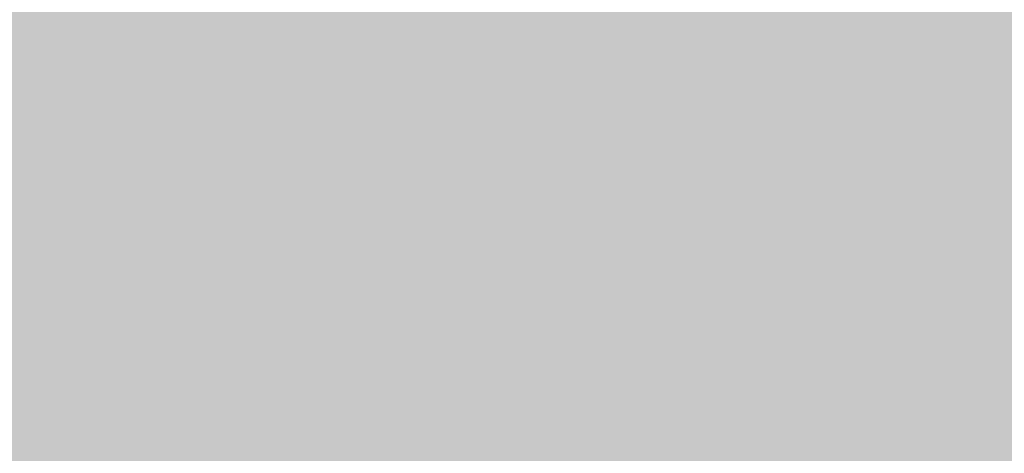
# Model space of a CAD drawing. Units: feet. Extents: x 3168 to 4724, y 827 to 1477.
# Tile 100 of 256: x 3277.376 to 3284.479, y 1093.654 to 1096.781. Entities that reach past the tile are written whole.
import ezdxf

# ---------------------------------------------------------------- set-up
doc = ezdxf.new("R2010")
doc.units = ezdxf.units.FT
doc.layers.add('A-ELEV-PATT', color=8, linetype='Continuous', lineweight=13)

msp = doc.modelspace()

# ---------------------------------------------------------------- hatches: boundary and pattern name
at = {"layer": 'A-ELEV-PATT'}
h = msp.add_hatch(color=256, dxfattribs=at)
h.dxf.hatch_style = 1
edge = h.paths.add_edge_path()
edge.add_ellipse((3552.9058, 979.2201), major_axis=(36.7449, 0), ratio=0.4848485, start_angle=0, end_angle=360)
edge = h.paths.add_edge_path()
edge.add_ellipse((3559.8916, 929.2523), major_axis=(36.7449, 0), ratio=0.4848485, start_angle=0, end_angle=360)
edge = h.paths.add_edge_path()
edge.add_line((3299.3168, 1198.6061), (3479.9167, 1198.6061))
edge.add_line((3479.9167, 1198.6061), (3479.9167, 1209.8686))
edge.add_spline(control_points=[(3479.9167, 1209.8686), (3464.3012, 1209.8686), (3448.6856, 1209.8686), (3410.9491, 1209.8686), (3388.8282, 1209.8686), (3355.6469, 1209.8686), (3344.5864, 1209.8686), (3327.9957, 1209.8686), (3322.4655, 1209.8686), (3314.1702, 1209.8686), (3311.4051, 1209.8686), (3307.2574, 1209.8686), (3305.8748, 1209.8686), (3303.801, 1209.8686), (3303.1097, 1209.8686), (3302.0728, 1209.8686), (3301.7272, 1209.8686), (3301.2087, 1209.8686), (3301.0359, 1209.8686), (3300.7767, 1209.8686), (3300.6903, 1209.8686), (3300.5606, 1209.8686), (3300.5174, 1209.8686), (3300.4526, 1209.8686), (3300.431, 1209.8686), (3300.3986, 1209.8686), (3300.3878, 1209.8686), (3300.3662, 1209.8686), (3300.3457, 1209.8686), (3300.3455, 1209.8686), (3300.3455, 1209.8686), (3300.3433, 1209.8686), (3300.3411, 1209.8686), (3300.3379, 1209.8686), (3300.3368, 1209.8686), (3300.3339, 1209.8686), (3300.3321, 1209.8686), (3300.3255, 1209.8686), (3300.3207, 1209.8686), (3300.3109, 1209.8686), (3300.306, 1209.8686), (3300.2905, 1209.8686), (3300.28, 1209.8686), (3300.2324, 1209.8688), (3300.1953, 1209.869), (3299.9511, 1209.8706), (3299.7448, 1209.8743), (3299.4368, 1209.8833), (3299.3344, 1209.8868), (3299.1811, 1209.8929), (3299.13, 1209.8951), (3298.6522, 1209.9168), (3298.2295, 1209.9457), (3297.6016, 1210.0024), (3297.3934, 1210.0235), (3297.0827, 1210.0583), (3296.9793, 1210.0705), (3296.293, 1210.1549), (3295.7181, 1210.2434), (3294.8687, 1210.3989), (3294.5877, 1210.4545), (3294.1693, 1210.5433), (3294.0304, 1210.5739), (3291.7071, 1211.1012), (3289.6536, 1211.8134), (3285.7763, 1213.564), (3283.9514, 1214.6035), (3280.5122, 1216.9801), (3278.8972, 1218.3176), (3276.3799, 1220.8295), (3275.416, 1221.9177), (3274.0393, 1223.7077), (3273.581, 1224.3495), (3273.1432, 1225.0163)], knot_values=[39.119033, 39.119033, 39.119033, 39.119033, 39.286353, 39.286353, 39.523379, 39.523379, 39.641892, 39.641892, 39.701148, 39.701148, 39.730777, 39.730777, 39.745591, 39.745591, 39.752998, 39.752998, 39.756701, 39.756701, 39.758553, 39.758553, 39.759479, 39.759479, 39.759942, 39.759942, 39.760173, 39.760173, 39.760289, 39.760289, 39.760405, 39.760405, 39.760463, 39.760463, 39.763389, 39.763389, 39.764851, 39.764851, 39.767304, 39.767304, 39.773825, 39.773825, 39.78057, 39.78057, 39.79477, 39.79477, 39.845194, 39.845194, 40.126715, 40.126715, 40.267476, 40.267476, 40.337856, 40.337856, 40.927023, 40.927023, 41.221606, 41.221606, 41.368898, 41.368898, 42.202622, 42.202622, 42.619485, 42.619485, 42.827916, 42.827916, 46.118323, 46.118323, 49.408731, 49.408731, 52.699139, 52.699139, 54.927489, 54.927489, 56.104228, 56.104228, 56.104228, 56.104228], weights=[1, 1, 1, 1, 1, 1, 1, 1, 1, 1, 1, 1, 1, 1, 1, 1, 1, 1, 1, 1, 1, 1, 1, 1, 1, 1, 1, 1, 1, 1, 1, 1, 1, 1, 1, 1, 1, 1, 1, 1, 1, 1, 1, 1, 1, 1, 1, 1, 1, 1, 1, 1, 1, 1, 1, 1, 1, 1, 1, 1, 1, 1, 1, 1, 1, 1, 1, 1, 1, 1, 1, 1, 1, 1], degree=3, periodic=0)
edge.add_line((3273.1432, 1225.0163), (3273.1432, 1099.0163))
edge.add_line((3273.1432, 1099.0163), (3299.3168, 1099.0163))
edge.add_line((3299.3168, 1099.0163), (3299.3168, 1198.6061))
edge = h.paths.add_edge_path()
edge.add_line((3304.7584, 1324.1581), (3479.9167, 1324.1581))
edge.add_line((3479.9167, 1324.1581), (3479.9167, 1335.7146))
edge.add_line((3479.9167, 1335.7146), (3269.1616, 1335.7146))
edge.add_spline(control_points=[(3269.1616, 1335.7146), (3264.0242, 1335.7146), (3258.3641, 1328.9582), (3259.2643, 1323.9003)], knot_values=[0, 0, 0, 0, 15.412191, 15.412191, 15.412191, 15.412191], degree=3, periodic=0)
edge.add_line((3259.2643, 1323.9003), (3265.5168, 1288.7691))
edge.add_line((3265.5168, 1288.7691), (3275.2651, 1261.5456))
edge.add_line((3275.2651, 1261.5456), (3304.7584, 1261.5456))
edge.add_line((3304.7584, 1261.5456), (3304.7584, 1324.1581))
h = msp.add_hatch(color=256, dxfattribs=at)
h.dxf.hatch_style = 1
h.paths.add_polyline_path([(3384.5252, 1099.0163), (3335.0292, 1099.0163), (3299.3168, 1099.0163), (3273.1432, 1099.0163), (3217.5654, 1099.0163), (3168.0693, 827.1163), (3335.0292, 827.1163)])

doc.saveas('drawing.dxf')
